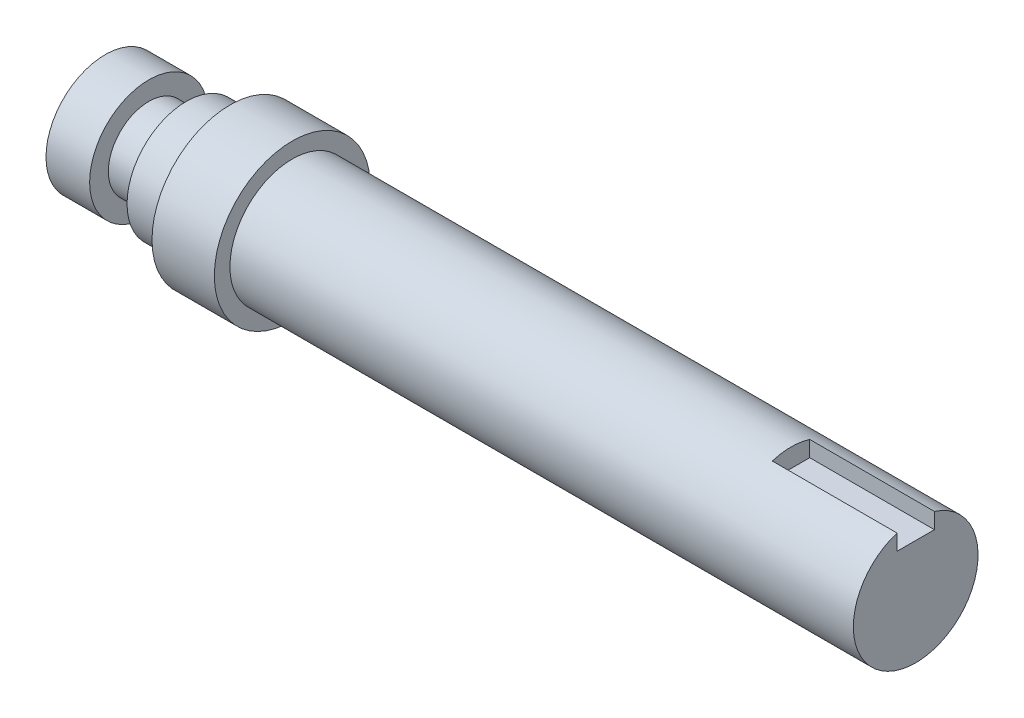
ISO-10303-21;
HEADER;
FILE_DESCRIPTION(('STEP AP214'),'2;1');
FILE_NAME('part.step','',(''),(''),'','','');
FILE_SCHEMA(('AUTOMOTIVE_DESIGN { 1 0 10303 214 1 1 1 1 }'));
ENDSEC;
DATA;
#1=APPLICATION_CONTEXT('core data for automotive mechanical design processes');
#2=APPLICATION_PROTOCOL_DEFINITION('international standard','automotive_design',2000,#1);
#3=PRODUCT_CONTEXT('',#1,'mechanical');
#4=PRODUCT('Part','Part','',(#3));
#5=PRODUCT_RELATED_PRODUCT_CATEGORY('part','',(#4));
#6=PRODUCT_DEFINITION_FORMATION('','',#4);
#7=PRODUCT_DEFINITION_CONTEXT('part definition',#1,'design');
#8=PRODUCT_DEFINITION('design','',#6,#7);
#9=PRODUCT_DEFINITION_SHAPE('','',#8);
#10=(LENGTH_UNIT() NAMED_UNIT(*) SI_UNIT(.MILLI.,.METRE.));
#11=(NAMED_UNIT(*) PLANE_ANGLE_UNIT() SI_UNIT($,.RADIAN.));
#12=(NAMED_UNIT(*) SI_UNIT($,.STERADIAN.) SOLID_ANGLE_UNIT());
#13=UNCERTAINTY_MEASURE_WITH_UNIT(LENGTH_MEASURE(1.E-05),#10,'distance_accuracy_value','');
#14=(GEOMETRIC_REPRESENTATION_CONTEXT(3) GLOBAL_UNCERTAINTY_ASSIGNED_CONTEXT((#13)) GLOBAL_UNIT_ASSIGNED_CONTEXT((#10,
#11,#12)) REPRESENTATION_CONTEXT('',''));
#15=CARTESIAN_POINT('',(0.,0.,0.));
#16=DIRECTION('',(0.,0.,1.));
#17=DIRECTION('',(1.,0.,0.));
#18=AXIS2_PLACEMENT_3D('',#15,#16,#17);
#19=CARTESIAN_POINT('',(0.,0.,0.));
#20=DIRECTION('',(-1.,0.,0.));
#21=DIRECTION('',(0.,0.,1.));
#22=AXIS2_PLACEMENT_3D('',#19,#20,#21);
#23=CYLINDRICAL_SURFACE('',#22,10.);
#24=CARTESIAN_POINT('',(30.,0.,0.));
#25=DIRECTION('',(-1.,0.,0.));
#26=DIRECTION('',(0.,0.,1.));
#27=AXIS2_PLACEMENT_3D('',#24,#25,#26);
#28=CIRCLE('',#27,10.);
#29=CARTESIAN_POINT('',(30.,0.,10.));
#30=VERTEX_POINT('',#29);
#31=EDGE_CURVE('E113',#30,#30,#28,.T.);
#32=ORIENTED_EDGE('',*,*,#31,.F.);
#33=EDGE_LOOP('',(#32));
#34=FACE_BOUND('',#33,.T.);
#35=DIRECTION('',(-1.,0.,0.));
#36=VECTOR('',#35,1.);
#37=CARTESIAN_POINT('',(0.,9.53939201416946,-3.));
#38=LINE('',#37,#36);
#39=CARTESIAN_POINT('',(130.,9.53939201416946,-3.));
#40=VERTEX_POINT('',#39);
#41=CARTESIAN_POINT('',(110.,9.53939201416946,-3.));
#42=VERTEX_POINT('',#41);
#43=EDGE_CURVE('E83',#40,#42,#38,.T.);
#44=ORIENTED_EDGE('',*,*,#43,.F.);
#45=CARTESIAN_POINT('',(130.,0.,0.));
#46=DIRECTION('',(-1.,0.,0.));
#47=DIRECTION('',(0.,0.,1.));
#48=AXIS2_PLACEMENT_3D('',#45,#46,#47);
#49=CIRCLE('',#48,10.);
#50=CARTESIAN_POINT('',(130.,9.53939201416946,3.));
#51=VERTEX_POINT('',#50);
#52=EDGE_CURVE('E109',#40,#51,#49,.T.);
#53=ORIENTED_EDGE('',*,*,#52,.T.);
#54=DIRECTION('',(-1.,0.,0.));
#55=VECTOR('',#54,1.);
#56=CARTESIAN_POINT('',(0.,9.53939201416946,3.));
#57=LINE('',#56,#55);
#58=CARTESIAN_POINT('',(110.,9.53939201416946,3.));
#59=VERTEX_POINT('',#58);
#60=EDGE_CURVE('E53',#51,#59,#57,.T.);
#61=ORIENTED_EDGE('',*,*,#60,.T.);
#62=CARTESIAN_POINT('',(110.,0.,0.));
#63=DIRECTION('',(-1.,0.,0.));
#64=DIRECTION('',(0.,0.,1.));
#65=AXIS2_PLACEMENT_3D('',#62,#63,#64);
#66=CIRCLE('',#65,10.);
#67=EDGE_CURVE('E11',#59,#42,#66,.T.);
#68=ORIENTED_EDGE('',*,*,#67,.T.);
#69=EDGE_LOOP('',(#44,#53,#61,#68));
#70=FACE_BOUND('',#69,.T.);
#71=ADVANCED_FACE('F39',(#34,#70),#23,.T.);
#72=CARTESIAN_POINT('',(130.,10.,0.));
#73=DIRECTION('',(-1.,0.,0.));
#74=DIRECTION('',(0.,0.,1.));
#75=AXIS2_PLACEMENT_3D('',#72,#73,#74);
#76=PLANE('',#75);
#77=DIRECTION('',(0.,1.,0.));
#78=VECTOR('',#77,1.);
#79=CARTESIAN_POINT('',(130.,7.,-3.));
#80=LINE('',#79,#78);
#81=CARTESIAN_POINT('',(130.,7.,-3.));
#82=VERTEX_POINT('',#81);
#83=EDGE_CURVE('E65',#82,#40,#80,.T.);
#84=ORIENTED_EDGE('',*,*,#83,.F.);
#85=DIRECTION('',(0.,0.,1.));
#86=VECTOR('',#85,1.);
#87=CARTESIAN_POINT('',(130.,7.,-3.));
#88=LINE('',#87,#86);
#89=CARTESIAN_POINT('',(130.,7.,3.));
#90=VERTEX_POINT('',#89);
#91=EDGE_CURVE('E98',#82,#90,#88,.T.);
#92=ORIENTED_EDGE('',*,*,#91,.T.);
#93=DIRECTION('',(0.,1.,0.));
#94=VECTOR('',#93,1.);
#95=CARTESIAN_POINT('',(130.,7.,3.));
#96=LINE('',#95,#94);
#97=EDGE_CURVE('E86',#90,#51,#96,.T.);
#98=ORIENTED_EDGE('',*,*,#97,.T.);
#99=ORIENTED_EDGE('',*,*,#52,.F.);
#100=EDGE_LOOP('',(#84,#92,#98,#99));
#101=FACE_BOUND('',#100,.T.);
#102=ADVANCED_FACE('F186',(#101),#76,.F.);
#103=CARTESIAN_POINT('',(0.,0.,0.));
#104=DIRECTION('',(1.,0.,0.));
#105=DIRECTION('',(0.,0.,-1.));
#106=AXIS2_PLACEMENT_3D('',#103,#104,#105);
#107=PLANE('',#106);
#108=CARTESIAN_POINT('',(0.,0.,0.));
#109=DIRECTION('',(-1.,0.,0.));
#110=DIRECTION('',(0.,0.,1.));
#111=AXIS2_PLACEMENT_3D('',#108,#109,#110);
#112=CIRCLE('',#111,9.5);
#113=CARTESIAN_POINT('',(0.,0.,9.5));
#114=VERTEX_POINT('',#113);
#115=EDGE_CURVE('E50',#114,#114,#112,.T.);
#116=ORIENTED_EDGE('',*,*,#115,.T.);
#117=EDGE_LOOP('',(#116));
#118=FACE_BOUND('',#117,.T.);
#119=ADVANCED_FACE('F41',(#118),#107,.F.);
#120=CARTESIAN_POINT('',(0.,0.,0.));
#121=DIRECTION('',(-1.,0.,0.));
#122=DIRECTION('',(0.,0.,1.));
#123=AXIS2_PLACEMENT_3D('',#120,#121,#122);
#124=CYLINDRICAL_SURFACE('',#123,9.5);
#125=ORIENTED_EDGE('',*,*,#115,.F.);
#126=EDGE_LOOP('',(#125));
#127=FACE_BOUND('',#126,.T.);
#128=CARTESIAN_POINT('',(7.,0.,0.));
#129=DIRECTION('',(-1.,0.,0.));
#130=DIRECTION('',(0.,0.,1.));
#131=AXIS2_PLACEMENT_3D('',#128,#129,#130);
#132=CIRCLE('',#131,9.5);
#133=CARTESIAN_POINT('',(7.,0.,9.5));
#134=VERTEX_POINT('',#133);
#135=EDGE_CURVE('E133',#134,#134,#132,.T.);
#136=ORIENTED_EDGE('',*,*,#135,.T.);
#137=EDGE_LOOP('',(#136));
#138=FACE_BOUND('',#137,.T.);
#139=ADVANCED_FACE('F139',(#127,#138),#124,.T.);
#140=CARTESIAN_POINT('',(7.,9.5,0.));
#141=DIRECTION('',(-1.,0.,0.));
#142=DIRECTION('',(0.,0.,1.));
#143=AXIS2_PLACEMENT_3D('',#140,#141,#142);
#144=PLANE('',#143);
#145=ORIENTED_EDGE('',*,*,#135,.F.);
#146=EDGE_LOOP('',(#145));
#147=FACE_BOUND('',#146,.T.);
#148=CARTESIAN_POINT('',(7.,0.,0.));
#149=DIRECTION('',(-1.,0.,0.));
#150=DIRECTION('',(0.,0.,1.));
#151=AXIS2_PLACEMENT_3D('',#148,#149,#150);
#152=CIRCLE('',#151,6.5);
#153=CARTESIAN_POINT('',(7.,0.,6.5));
#154=VERTEX_POINT('',#153);
#155=EDGE_CURVE('E134',#154,#154,#152,.T.);
#156=ORIENTED_EDGE('',*,*,#155,.T.);
#157=EDGE_LOOP('',(#156));
#158=FACE_BOUND('',#157,.T.);
#159=ADVANCED_FACE('F141',(#147,#158),#144,.F.);
#160=CARTESIAN_POINT('',(0.,0.,0.));
#161=DIRECTION('',(-1.,0.,0.));
#162=DIRECTION('',(0.,0.,1.));
#163=AXIS2_PLACEMENT_3D('',#160,#161,#162);
#164=CYLINDRICAL_SURFACE('',#163,6.5);
#165=ORIENTED_EDGE('',*,*,#155,.F.);
#166=EDGE_LOOP('',(#165));
#167=FACE_BOUND('',#166,.T.);
#168=CARTESIAN_POINT('',(13.,0.,0.));
#169=DIRECTION('',(-1.,0.,0.));
#170=DIRECTION('',(0.,0.,1.));
#171=AXIS2_PLACEMENT_3D('',#168,#169,#170);
#172=CIRCLE('',#171,6.5);
#173=CARTESIAN_POINT('',(13.,0.,6.5));
#174=VERTEX_POINT('',#173);
#175=EDGE_CURVE('E129',#174,#174,#172,.T.);
#176=ORIENTED_EDGE('',*,*,#175,.T.);
#177=EDGE_LOOP('',(#176));
#178=FACE_BOUND('',#177,.T.);
#179=ADVANCED_FACE('F149',(#167,#178),#164,.T.);
#180=CARTESIAN_POINT('',(13.,6.5,0.));
#181=DIRECTION('',(1.,0.,0.));
#182=DIRECTION('',(0.,0.,-1.));
#183=AXIS2_PLACEMENT_3D('',#180,#181,#182);
#184=PLANE('',#183);
#185=ORIENTED_EDGE('',*,*,#175,.F.);
#186=EDGE_LOOP('',(#185));
#187=FACE_BOUND('',#186,.T.);
#188=CARTESIAN_POINT('',(13.,0.,0.));
#189=DIRECTION('',(-1.,0.,0.));
#190=DIRECTION('',(0.,0.,1.));
#191=AXIS2_PLACEMENT_3D('',#188,#189,#190);
#192=CIRCLE('',#191,9.5);
#193=CARTESIAN_POINT('',(13.,0.,9.5));
#194=VERTEX_POINT('',#193);
#195=EDGE_CURVE('E123',#194,#194,#192,.T.);
#196=ORIENTED_EDGE('',*,*,#195,.T.);
#197=EDGE_LOOP('',(#196));
#198=FACE_BOUND('',#197,.T.);
#199=ADVANCED_FACE('F153',(#187,#198),#184,.F.);
#200=CARTESIAN_POINT('',(0.,0.,0.));
#201=DIRECTION('',(-1.,0.,0.));
#202=DIRECTION('',(0.,0.,1.));
#203=AXIS2_PLACEMENT_3D('',#200,#201,#202);
#204=CYLINDRICAL_SURFACE('',#203,9.5);
#205=ORIENTED_EDGE('',*,*,#195,.F.);
#206=EDGE_LOOP('',(#205));
#207=FACE_BOUND('',#206,.T.);
#208=CARTESIAN_POINT('',(20.,0.,0.));
#209=DIRECTION('',(-1.,0.,0.));
#210=DIRECTION('',(0.,0.,1.));
#211=AXIS2_PLACEMENT_3D('',#208,#209,#210);
#212=CIRCLE('',#211,9.5);
#213=CARTESIAN_POINT('',(20.,0.,9.5));
#214=VERTEX_POINT('',#213);
#215=EDGE_CURVE('E125',#214,#214,#212,.T.);
#216=ORIENTED_EDGE('',*,*,#215,.T.);
#217=EDGE_LOOP('',(#216));
#218=FACE_BOUND('',#217,.T.);
#219=ADVANCED_FACE('F159',(#207,#218),#204,.T.);
#220=CARTESIAN_POINT('',(20.,9.5,0.));
#221=DIRECTION('',(1.,0.,0.));
#222=DIRECTION('',(0.,0.,-1.));
#223=AXIS2_PLACEMENT_3D('',#220,#221,#222);
#224=PLANE('',#223);
#225=ORIENTED_EDGE('',*,*,#215,.F.);
#226=EDGE_LOOP('',(#225));
#227=FACE_BOUND('',#226,.T.);
#228=CARTESIAN_POINT('',(20.,0.,0.));
#229=DIRECTION('',(-1.,0.,0.));
#230=DIRECTION('',(0.,0.,1.));
#231=AXIS2_PLACEMENT_3D('',#228,#229,#230);
#232=CIRCLE('',#231,12.5);
#233=CARTESIAN_POINT('',(20.,0.,12.5));
#234=VERTEX_POINT('',#233);
#235=EDGE_CURVE('E118',#234,#234,#232,.T.);
#236=ORIENTED_EDGE('',*,*,#235,.T.);
#237=EDGE_LOOP('',(#236));
#238=FACE_BOUND('',#237,.T.);
#239=ADVANCED_FACE('F168',(#227,#238),#224,.F.);
#240=CARTESIAN_POINT('',(0.,0.,0.));
#241=DIRECTION('',(-1.,0.,0.));
#242=DIRECTION('',(0.,0.,1.));
#243=AXIS2_PLACEMENT_3D('',#240,#241,#242);
#244=CYLINDRICAL_SURFACE('',#243,12.5);
#245=ORIENTED_EDGE('',*,*,#235,.F.);
#246=EDGE_LOOP('',(#245));
#247=FACE_BOUND('',#246,.T.);
#248=CARTESIAN_POINT('',(30.,0.,0.));
#249=DIRECTION('',(-1.,0.,0.));
#250=DIRECTION('',(0.,0.,1.));
#251=AXIS2_PLACEMENT_3D('',#248,#249,#250);
#252=CIRCLE('',#251,12.5);
#253=CARTESIAN_POINT('',(30.,0.,12.5));
#254=VERTEX_POINT('',#253);
#255=EDGE_CURVE('E116',#254,#254,#252,.T.);
#256=ORIENTED_EDGE('',*,*,#255,.T.);
#257=EDGE_LOOP('',(#256));
#258=FACE_BOUND('',#257,.T.);
#259=ADVANCED_FACE('F175',(#247,#258),#244,.T.);
#260=CARTESIAN_POINT('',(30.,12.5,0.));
#261=DIRECTION('',(-1.,0.,0.));
#262=DIRECTION('',(0.,0.,1.));
#263=AXIS2_PLACEMENT_3D('',#260,#261,#262);
#264=PLANE('',#263);
#265=ORIENTED_EDGE('',*,*,#255,.F.);
#266=EDGE_LOOP('',(#265));
#267=FACE_BOUND('',#266,.T.);
#268=ORIENTED_EDGE('',*,*,#31,.T.);
#269=EDGE_LOOP('',(#268));
#270=FACE_BOUND('',#269,.T.);
#271=ADVANCED_FACE('F178',(#267,#270),#264,.F.);
#272=CARTESIAN_POINT('',(110.,7.,-3.));
#273=DIRECTION('',(-1.,0.,0.));
#274=DIRECTION('',(0.,0.,1.));
#275=AXIS2_PLACEMENT_3D('',#272,#273,#274);
#276=PLANE('',#275);
#277=DIRECTION('',(0.,-1.,0.));
#278=VECTOR('',#277,1.);
#279=CARTESIAN_POINT('',(110.,7.,3.));
#280=LINE('',#279,#278);
#281=CARTESIAN_POINT('',(110.,7.,3.));
#282=VERTEX_POINT('',#281);
#283=EDGE_CURVE('E95',#59,#282,#280,.T.);
#284=ORIENTED_EDGE('',*,*,#283,.T.);
#285=DIRECTION('',(0.,0.,1.));
#286=VECTOR('',#285,1.);
#287=CARTESIAN_POINT('',(110.,7.,-3.));
#288=LINE('',#287,#286);
#289=CARTESIAN_POINT('',(110.,7.,-3.));
#290=VERTEX_POINT('',#289);
#291=EDGE_CURVE('E87',#290,#282,#288,.T.);
#292=ORIENTED_EDGE('',*,*,#291,.F.);
#293=DIRECTION('',(0.,-1.,0.));
#294=VECTOR('',#293,1.);
#295=CARTESIAN_POINT('',(110.,7.,-3.));
#296=LINE('',#295,#294);
#297=EDGE_CURVE('E78',#42,#290,#296,.T.);
#298=ORIENTED_EDGE('',*,*,#297,.F.);
#299=ORIENTED_EDGE('',*,*,#67,.F.);
#300=EDGE_LOOP('',(#284,#292,#298,#299));
#301=FACE_BOUND('',#300,.T.);
#302=ADVANCED_FACE('F91',(#301),#276,.F.);
#303=CARTESIAN_POINT('',(0.,0.,-3.));
#304=DIRECTION('',(0.,0.,1.));
#305=DIRECTION('',(1.,0.,0.));
#306=AXIS2_PLACEMENT_3D('',#303,#304,#305);
#307=PLANE('',#306);
#308=ORIENTED_EDGE('',*,*,#43,.T.);
#309=ORIENTED_EDGE('',*,*,#297,.T.);
#310=DIRECTION('',(1.,0.,0.));
#311=VECTOR('',#310,1.);
#312=CARTESIAN_POINT('',(130.,7.,-3.));
#313=LINE('',#312,#311);
#314=EDGE_CURVE('E81',#290,#82,#313,.T.);
#315=ORIENTED_EDGE('',*,*,#314,.T.);
#316=ORIENTED_EDGE('',*,*,#83,.T.);
#317=EDGE_LOOP('',(#308,#309,#315,#316));
#318=FACE_BOUND('',#317,.T.);
#319=ADVANCED_FACE('F85',(#318),#307,.T.);
#320=CARTESIAN_POINT('',(0.,0.,3.));
#321=DIRECTION('',(0.,0.,1.));
#322=DIRECTION('',(1.,0.,0.));
#323=AXIS2_PLACEMENT_3D('',#320,#321,#322);
#324=PLANE('',#323);
#325=ORIENTED_EDGE('',*,*,#97,.F.);
#326=DIRECTION('',(1.,0.,0.));
#327=VECTOR('',#326,1.);
#328=CARTESIAN_POINT('',(130.,7.,3.));
#329=LINE('',#328,#327);
#330=EDGE_CURVE('E104',#282,#90,#329,.T.);
#331=ORIENTED_EDGE('',*,*,#330,.F.);
#332=ORIENTED_EDGE('',*,*,#283,.F.);
#333=ORIENTED_EDGE('',*,*,#60,.F.);
#334=EDGE_LOOP('',(#325,#331,#332,#333));
#335=FACE_BOUND('',#334,.T.);
#336=ADVANCED_FACE('F194',(#335),#324,.F.);
#337=CARTESIAN_POINT('',(130.,7.,-3.));
#338=DIRECTION('',(0.,-1.,0.));
#339=DIRECTION('',(1.,0.,0.));
#340=AXIS2_PLACEMENT_3D('',#337,#338,#339);
#341=PLANE('',#340);
#342=ORIENTED_EDGE('',*,*,#330,.T.);
#343=ORIENTED_EDGE('',*,*,#91,.F.);
#344=ORIENTED_EDGE('',*,*,#314,.F.);
#345=ORIENTED_EDGE('',*,*,#291,.T.);
#346=EDGE_LOOP('',(#342,#343,#344,#345));
#347=FACE_BOUND('',#346,.T.);
#348=ADVANCED_FACE('F96',(#347),#341,.F.);
#349=CLOSED_SHELL('',(#71,#102,#119,#139,#159,#179,#199,#219,#239,#259,#271,#302,#319,#336,#348));
#350=MANIFOLD_SOLID_BREP('B2',#349);
#351=ADVANCED_BREP_SHAPE_REPRESENTATION('',(#18,#350),#14);
#352=SHAPE_DEFINITION_REPRESENTATION(#9,#351);
ENDSEC;
END-ISO-10303-21;
